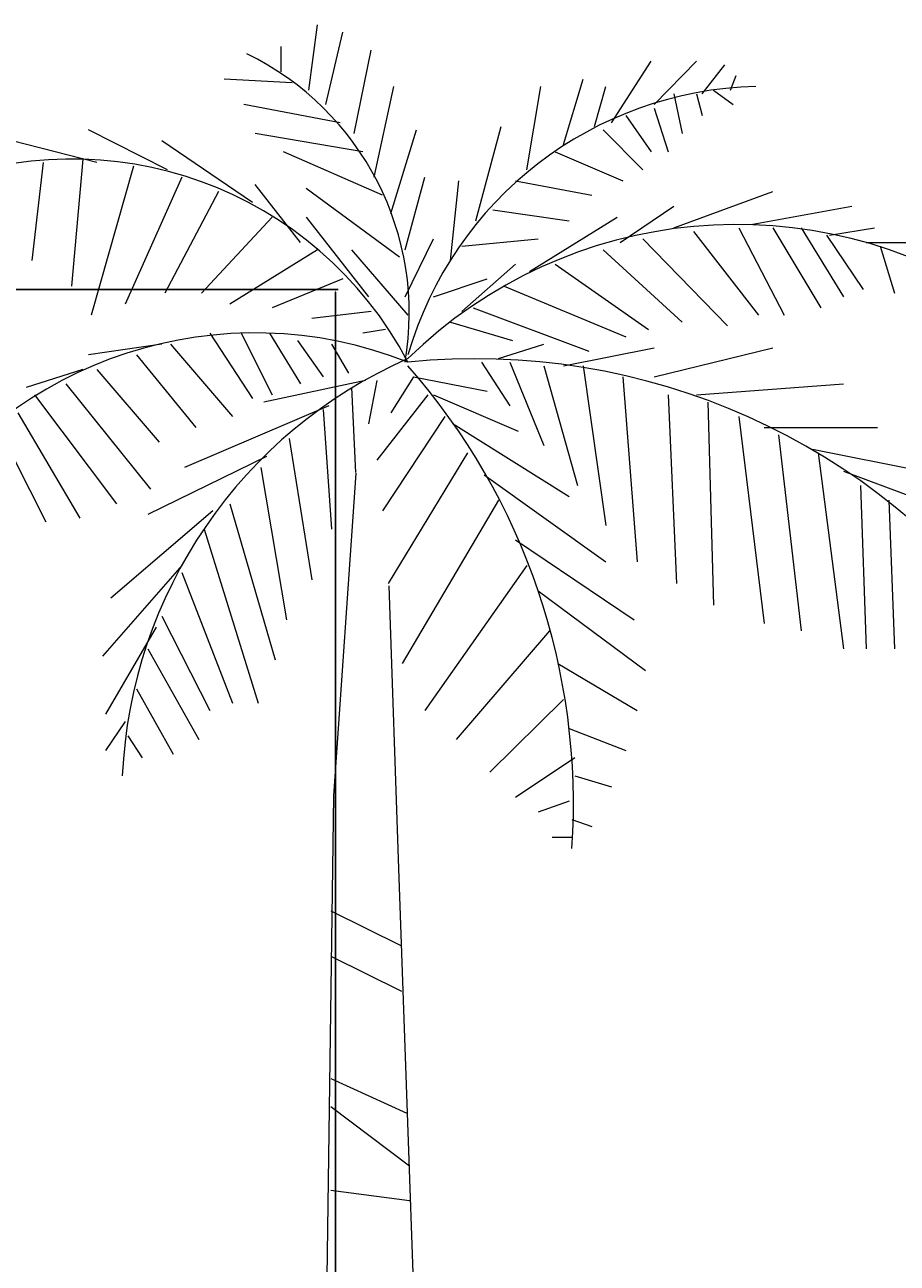
# Model space of a CAD drawing. Units: inches. Extents: x -301 to 715, y -607 to 364.
# Tile 136 of 141: x 194 to 254, y -391 to -306. Entities that reach past the tile are written whole.
import ezdxf

# ---------------------------------------------------------------- set-up
doc = ezdxf.new("R2010")
doc.units = ezdxf.units.IN
doc.header["$MEASUREMENT"] = 0
doc.layers.add('A-ANNO-DIMS', color=2, linetype='Continuous', lineweight=18)
doc.layers.add('L-PLNT', color=94, linetype='Continuous', lineweight=13)
doc.styles.get("Standard").update_dxf_attribs({"font": 'arial.ttf'})
doc.dimstyles.get("Standard").update_dxf_attribs({"dimtxt": 0.18, "dimasz": 0.18, "dimexe": 0.18, "dimexo": 0.0625, "dimgap": 0.09, "dimtad": 0, "dimtih": 1, "dimtoh": 1, "dimdec": 1, "dimzin": 0, "dimdsep": 46, "dimlunit": 4, "dimtxsty": 'Standard', "dimcen": 0.09, "dimclrd": 3, "dimclre": 4, "dimclrt": 6, "dimadec": 0, "dimazin": 0, "dimtfac": 1, "dimtdec": 1, "dimtofl": 0, "dimtmove": 0, "dimatfit": 3, "dimfxl": 1, "dimtfill": 2, "dimtfillclr": 51, "dimtolj": 1, "dimtzin": 0, "dimarcsym": 0})

# ---------------------------------------------------------------- blocks, each defined once
blk = doc.blocks.new('*U34')
for p, q in [((-5.567, 196.707), (-4.987, 201.167)), ((-4.407, 195.716), (-3.247, 200.672)), ((-7.5, 199.68), (-7.5, 197.946)), ((-2.474, 193.733), (-1.315, 199.433)), ((15.116, 194.477), (17.822, 198.689)), ((18.015, 195.716), (20.914, 198.689)), ((21.301, 196.459), (22.847, 198.441)), ((-6.727, 197.202), (-11.366, 197.45)), ((11.829, 192.99), (13.182, 197.45)), ((23.234, 196.707), (23.62, 197.698)), ((-1.121, 190.759), (0.232, 196.955)), ((9.317, 191.255), (10.283, 196.955)), ((13.956, 194.229), (14.729, 196.955)), ((19.368, 196.459), (19.948, 193.733)), ((20.914, 196.459), (21.301, 194.972)), ((22.074, 196.707), (23.427, 195.716)), ((-3.441, 194.477), (-10.013, 195.716)), ((18.015, 195.468), (18.981, 192.494)), ((16.082, 194.972), (17.822, 192.494)), ((-15.232, 191.255), (-20.644, 193.981)), ((-1.894, 192.494), (-9.24, 193.733)), ((0.038, 188.281), (1.778, 193.981)), ((5.837, 187.786), (7.577, 194.229)), ((14.536, 193.981), (17.242, 191.255)), ((-20.064, 191.751), (-25.863, 193.238)), ((-9.433, 189.025), (-15.618, 193.238)), ((-0.541, 189.52), (-7.307, 192.494)), ((11.25, 192.494), (15.889, 190.512)), ((-23.737, 191.751), (-24.51, 185.06)), ((-21.031, 191.998), (-21.804, 183.325)), ((-17.551, 191.503), (-20.451, 181.343)), ((-14.265, 190.759), (-18.131, 182.086)), ((1.005, 185.803), (2.358, 190.759)), ((4.098, 185.06), (4.678, 190.512)), ((8.544, 190.512), (13.763, 189.52)), ((-11.753, 189.768), (-15.425, 182.83)), ((-6.147, 186.299), (-9.24, 190.264)), ((-5.76, 190.016), (0.618, 185.308)), ((19.368, 187.29), (26.133, 189.768)), ((15.695, 186.299), (19.368, 188.777)), ((24.78, 187.538), (31.546, 188.777)), ((-8.08, 188.034), (-12.912, 182.83)), ((-5.76, 188.034), (-1.508, 182.582)), ((6.997, 188.529), (12.216, 187.786)), ((9.51, 184.317), (15.502, 188.034)), ((20.721, 187.042), (25.167, 181.343)), ((23.814, 187.29), (26.907, 181.343)), ((26.133, 187.29), (29.419, 181.838)), ((28.066, 187.29), (30.966, 182.582)), ((29.999, 186.795), (33.092, 187.29)), ((1.005, 182.582), (2.938, 186.547)), ((4.871, 186.051), (10.09, 186.547)), ((17.242, 186.547), (23.041, 180.599)), ((29.806, 186.795), (32.319, 183.078)), ((32.512, 186.299), (35.218, 186.299)), ((-4.987, 185.803), (-10.979, 182.086)), ((-2.668, 185.803), (1.198, 181.343)), ((14.536, 185.803), (19.948, 180.847)), ((33.479, 186.051), (34.445, 182.83)), ((4.871, 181.591), (8.544, 184.812)), ((11.25, 184.812), (17.628, 180.352)), ((-3.247, 183.821), (-8.08, 181.838)), ((2.938, 182.582), (6.61, 183.821)), ((7.77, 183.325), (16.082, 179.856)), ((-1.315, 181.591), (-5.374, 181.095)), ((5.644, 181.838), (13.569, 178.865)), ((-0.348, 180.352), (-1.894, 180.104)), ((4.098, 180.847), (8.35, 179.608)), ((-15.618, 179.36), (-20.644, 178.617)), ((-15.038, 179.36), (-10.786, 174.404)), ((-12.332, 180.104), (-9.433, 175.643)), ((-10.206, 180.104), (-8.08, 175.891)), ((-8.273, 180.104), (-6.147, 176.635)), ((-6.34, 179.608), (-4.6, 177.13)), ((-4.021, 179.36), (-2.861, 177.378)), ((7.384, 178.369), (10.476, 179.36)), ((-17.358, 178.617), (-13.299, 173.661)), ((11.829, 177.874), (18.015, 179.113)), ((18.015, 177.13), (26.133, 179.113)), ((-21.031, 177.626), (-24.897, 176.387)), ((-20.064, 177.626), (-15.812, 172.67)), ((6.224, 178.121), (8.157, 175.148)), ((8.157, 178.121), (10.476, 172.422)), ((10.476, 177.874), (12.796, 169.696)), ((13.182, 177.874), (14.729, 166.97)), ((-1.701, 176.882), (-8.66, 175.396)), ((-0.928, 176.882), (-1.508, 173.909)), ((1.585, 177.13), (0.038, 174.652)), ((1.585, 177.13), (6.61, 176.139)), ((15.889, 177.13), (16.855, 164.492)), ((-22.191, 176.635), (-16.391, 169.448)), ((-2.668, 176.387), (-2.376, 170.594)), ((20.914, 175.891), (30.966, 176.635)), ((-24.317, 175.891), (-18.711, 168.457)), ((-4.214, 175.148), (-14.072, 170.935)), ((2.551, 175.891), (-0.928, 171.431)), ((2.938, 175.891), (8.737, 173.413)), ((18.981, 175.891), (19.561, 163.005)), ((21.688, 175.396), (22.074, 161.518)), ((-25.476, 174.652), (-21.224, 167.466)), ((-4.6, 174.9), (-4.021, 166.722)), ((3.711, 174.404), (-0.541, 167.961)), ((23.814, 174.404), (25.554, 160.279)), ((-26.829, 173.661), (-23.544, 167.218)), ((4.291, 173.909), (12.216, 168.953)), ((25.554, 173.661), (33.285, 173.661)), ((-6.92, 172.917), (-5.374, 163.253)), ((26.52, 173.165), (28.066, 159.784)), ((5.257, 171.926), (-0.155, 163.005)), ((28.839, 172.174), (36.378, 170.687)), ((29.226, 171.926), (30.966, 158.545)), ((-8.466, 171.678), (-16.585, 167.713)), ((-8.853, 170.935), (-7.113, 160.527)), ((6.417, 170.439), (14.729, 164.492)), ((30.966, 170.687), (38.891, 167.713)), ((32.126, 169.696), (32.512, 158.545)), ((-10.979, 168.457), (-7.887, 157.801)), ((7.384, 168.705), (0.812, 157.553)), ((34.058, 168.705), (34.445, 158.545)), ((-12.139, 167.961), (-19.098, 162.014)), ((-12.719, 166.722), (-9.046, 154.828)), ((8.544, 165.979), (16.662, 160.527)), ((-14.265, 164.244), (-19.678, 158.049)), ((9.317, 164.244), (2.358, 154.332)), ((-14.265, 163.749), (-10.786, 154.828)), ((10.09, 162.51), (17.435, 157.058)), ((-15.618, 160.775), (-12.332, 154.332)), ((-16.005, 160.031), (-19.484, 154.084)), ((10.863, 159.784), (4.484, 152.35)), ((-16.585, 158.545), (-13.106, 152.35)), ((11.443, 157.553), (16.855, 154.332)), ((-17.358, 155.819), (-14.845, 151.358)), ((11.829, 155.075), (6.804, 150.119)), ((-18.131, 153.589), (-19.484, 151.606)), ((-17.938, 152.597), (-16.972, 151.111)), ((12.216, 153.093), (16.082, 151.606)), ((12.603, 151.111), (8.544, 148.385)), ((12.603, 149.872), (15.116, 149.128)), ((12.216, 148.137), (10.09, 147.393)), ((12.409, 146.898), (13.763, 146.402)), ((12.409, 145.659), (11.056, 145.659)), ((-4.081, 140.645), (0.753, 138.261)), ((-4.081, 137.547), (0.753, 135.163)), ((-4.081, 129.205), (1.124, 126.821)), ((-4.081, 127.298), (1.31, 123.246)), ((-4.081, 121.578), (1.31, 120.863))]:
    blk.add_line(p, q)
for points in [[(-2.363, 170.553), (-3.88, 148.505), (-4.988, 69.634), (-3.325, 24.869), (0, 0)], [(-0.116, 162.848), (0.554, 143.532), (2.217, 96.635), (3.88, 44.054), (7.76, 12.079), (11.64, 0)]]:
    blk.add_lwpolyline(points)
for centre, radius, start, end in [((-18.427, 181.448), 19.715, 350.285, 64.11229), ((25.595, 171.567), 25.395, 91.40319, 163.882), ((-21.738, 166.094), 25.899, 27.67115, 112.5305), ((23.687, 155.341), 32.188, 56.19272, 134.3213), ((-9.259, 151.732), 28.386, 68.38311, 147.5322), ((14.394, 148.393), 32.752, 113.7592, 177.4133), ((5.828, 132.718), 45.639, 35.98777, 95.82273), ((-32.8, 147.923), 45.309, 356.1943, 41.37848)]:
    blk.add_arc(centre, radius, start, end)
blk = doc.blocks.new('*D176')
at = {"layer": 'A-ANNO-DIMS', "color": 4, "lineweight": -2, "transparency": 16777216}
for p, q in [((148.28, -324.477), (215.605, -324.477)), ((-15.22, -540.477), (215.605, -540.477))]:
    blk.add_line(p, q, dxfattribs=at)
at = {"layer": 'A-ANNO-DIMS', "color": 3, "lineweight": -2, "transparency": 16777216}
for p, q in [((215.425, -324.657), (215.425, -432.296)), ((215.425, -540.297), (215.425, -432.659))]:
    blk.add_line(p, q, dxfattribs=at)
at = {"layer": 'A-ANNO-DIMS', "color": 3, "transparency": 16777216}
for points in [[(215.395, -324.657), (215.455, -324.657), (215.425, -324.477)], [(215.395, -540.297), (215.455, -540.297), (215.425, -540.477)]]:
    blk.add_solid(points, dxfattribs=at)
at = {"layer": 'Defpoints', "color": 0, "transparency": 16777216}
for p in [(148.218, -324.477), (-15.282, -540.477), (215.425, -540.477)]:
    blk.add_point(p, dxfattribs=at)
at = {"layer": 'A-ANNO-DIMS', "color": 6, "transparency": 16777216, "insert": (215.425, -432.477), "char_height": 0.18, "attachment_point": 5, "bg_fill": 1, "box_fill_scale": 1.25, "bg_fill_color": 51, "bg_fill_transparency": 0}
blk.add_mtext('\\A1;18\'-0"', dxfattribs=at)

msp = doc.modelspace()

# ---------------------------------------------------------------- block references
at = {"layer": 'L-PLNT'}
msp.add_blockref('*U34', (219.184, -507.552), dxfattribs=at)

# ---------------------------------------------------------------- dimensions: what is measured, and where the dimension line sits
at = {"layer": 'A-ANNO-DIMS'}
dim = msp.add_linear_dim(base=(215.425, -540.477), p1=(148.218, -324.477), p2=(-15.282, -540.477), angle=90, dimstyle='Standard', override={"dimdec": 1, "dimlfac": 1, "dimrnd": 0, "dimzin": 1, "dimdsep": 46, "dimlunit": 4, "dimfrac": 2}, dxfattribs=at)
dim.commit()
dim.dimension.update_dxf_attribs({"geometry": '*D176', "text_midpoint": (215.425, -432.477)})

doc.saveas('drawing.dxf')
